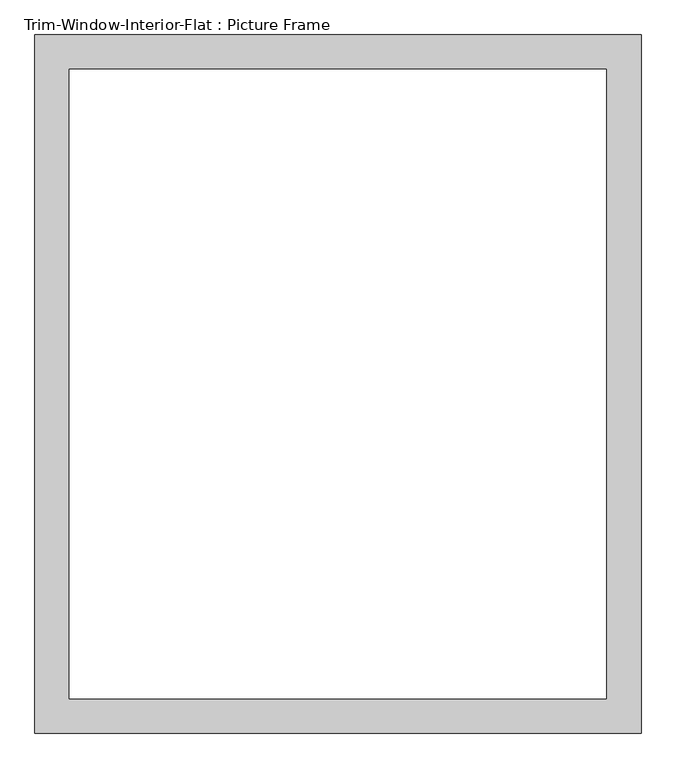
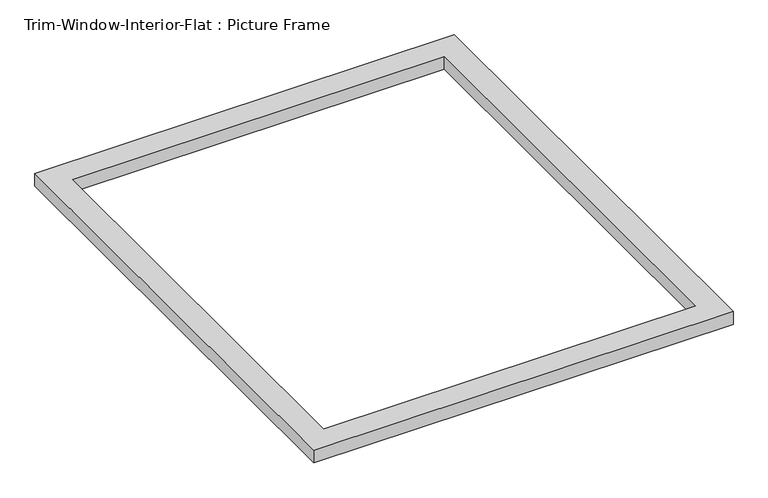
"""IFC4 building model written with IfcOpenShell, lengths in millimetres: proxy geometry, Trim-Window-Interior-Flat : Picture Frame."""

from ifc_helpers import new_model, si_unit, origin, origin_with_axes, place, context, project, spatial, polyline, outline, extrude, source, transform, mapped, element, save


def trim_window_interior_flat_picture_frame_dc353545(model_context):
    return source(origin(), model_context, "Body", "SweptSolid", [
        extrude(outline(polyline([(501.65, 44.45), (501.65, -1111.25), (-501.65, -1111.25), (-501.65, 44.45), (501.65, 44.45)]), holes=[polyline([(444.5, -12.7), (-444.5, -12.7), (-444.5, -1054.1), (444.5, -1054.1), (444.5, -12.7)])]), origin_with_axes(), (0.0, 0.0, 1.0), 31.75),
    ])


if __name__ == "__main__":
    model = new_model("IFC4")
    model_context = context("Model", 3, world=origin())
    ifc_project = project(units=[si_unit("LENGTHUNIT", "METRE", prefix="MILLI")], contexts=[model_context])
    site = spatial("IfcSite", under=ifc_project)
    building = spatial("IfcBuilding", under=site)
    placement = place(None, origin())
    trim_window_interior_flat_picture_frame_shape = trim_window_interior_flat_picture_frame_dc353545(model_context)
    element("IfcBuildingElementProxy", 1, Name="Trim-Window-Interior-Flat : Picture Frame", ObjectType="Trim-Window-Interior-Flat : Picture Frame", at=placement, inside=building, context=model_context, shape_type="MappedRepresentation", body=[
        mapped(trim_window_interior_flat_picture_frame_shape, transform((0.0, 0.0, 0.0), x_axis=(1.0, 0.0, 0.0), y_axis=(0.0, 1.0, 0.0), z_axis=(0.0, 0.0, 1.0))),
    ])
    save(model, "model.ifc")

# Revit data of these elements
# Type "Trim-Window-Interior-Flat : Picture Frame"
#   Trim Thickness_Picture Frame = 0' - 1 1/4"
#   Trim Width = 0' - 2 1/4"
#   Trim Thickness_with Sill = 0' - 0 3/4"
#   Sill Thickness = 0' - 1 1/4"
#   Opening Width [instance default] = 2' - 0"
#   Opening Height [instance default] = 3' - 0"
#   Default Elevation = 4' - 0"
#   Sill = no
#   Picture Frame = yes
#   Trim Material [instance default] = none
# Element 1 (IfcBuildingElementProxy, "Trim-Window-Interior-Flat : Picture Frame")
#   Opening Width = 3' - 0"
#   Opening Height = 3' - 6"
#   Trim Material = Wood - Stained
#   Materials on its faces: "Wood - Stained"
# Materials
#   "Wood - Stained": class "Wood", colour RGB 224 178 126, transparency 0, Cost = 0
